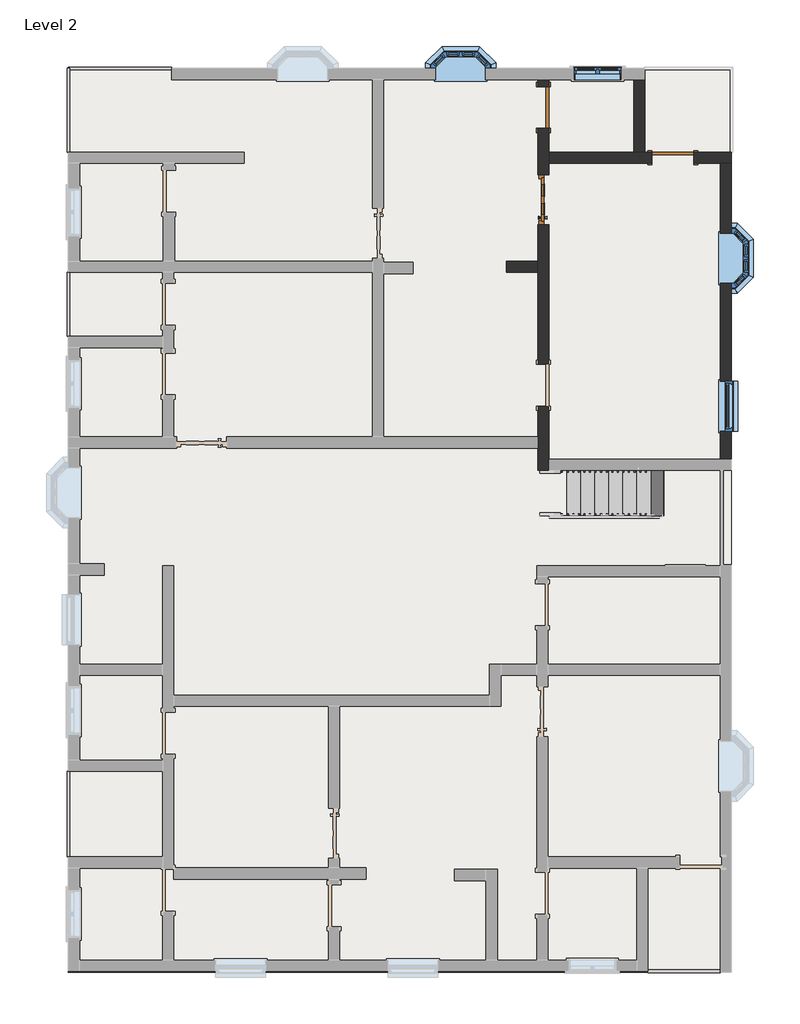
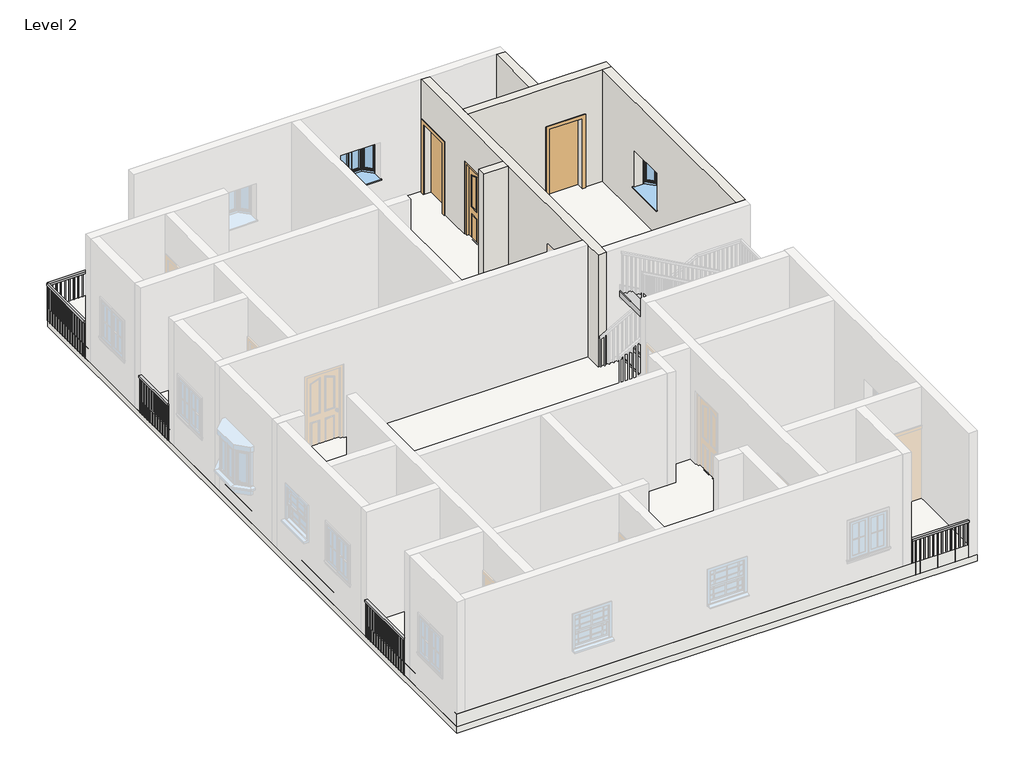
# One storey, part 2 of 4: 5 railings, 5 walls, 4 windows, 3 doors, 1 roof, 1 slab, 1 stair flight.
"""IFC4 building model written with IfcOpenShell, lengths in millimetres."""

from ifc_helpers import new_model, si_unit, frame, origin, place, context, project, spatial, polyline, outline, extrude, faceted_brep, transform, mapped, element, save
from components import doors_extsgl_12_910x2110mm_9a09825e, door_53b1b562, stair_flight_04592867, window_910x910mm_67ef725a, window_c29befe5, windows_sash_w_bars_1_910x910mm_b688f793

model = new_model("IFC4")

# Units and contexts
model_context = context("Model", 3, world=origin())
ifc_project = project(units=[si_unit("LENGTHUNIT", "METRE", prefix="MILLI")], contexts=[model_context])

# Site, building, storey
site = spatial("IfcSite", under=ifc_project)
building = spatial("IfcBuilding", under=site)
storey = spatial("IfcBuildingStorey", under=building, Name="Level 2", Elevation=3048.0)

# Doors
placement = place(None, origin())
doors_extsgl_12_910x2110mm_shape = doors_extsgl_12_910x2110mm_9a09825e(model_context)
element("IfcDoor", 1, ObjectType="Doors_ExtSgl_12 : 910x2110mm", at=placement, inside=storey, context=model_context, shape_type="MappedRepresentation", body=[
    mapped(doors_extsgl_12_910x2110mm_shape, transform((1600.6941283, 5934.0547293, 3048.0), x_axis=(0.0, 1.0, 0.0), y_axis=(-1.0, 0.0, 0.0), z_axis=(0.0, 0.0, 1.0))),
])
door_shape = door_53b1b562(model_context)
element("IfcDoor", 2, ObjectType="Single-Flush : 30\" x 80\"", at=placement, inside=storey, context=model_context, shape_type="MappedRepresentation", body=[
    mapped(door_shape, transform((1600.6941283, 7610.4547293, 3048.0), x_axis=(0.0, 1.0, 0.0), y_axis=(-1.0, 0.0, 0.0), z_axis=(0.0, 0.0, 1.0))),
])
element("IfcDoor", 3, ObjectType="Single-Flush : 30\" x 80\"", at=placement, inside=storey, context=model_context, shape_type="MappedRepresentation", body=[
    mapped(door_shape, transform((3962.8941283, 6696.0547293, 3048.0), x_axis=(-1.0, 0.0, 0.0), y_axis=(0.0, -1.0, 0.0), z_axis=(0.0, 0.0, 1.0))),
])

# Railings
element("IfcRailing", 4, ObjectType="Handrail - Rectangular", at=placement, inside=storey, context=model_context, shape_type="SweptSolid", body=[
    extrude(outline(polyline([(-7073.4058717, 4609.0339901), (-7022.6058717, 4609.0339901), (-7022.6058717, 3444.8547293), (-7073.4058717, 3444.8547293), (-7073.4058717, 4609.0339901)])), frame((0.0, 0.0, 3911.6), z_axis=(0.0, 0.0, 1.0), x_axis=(1.0, 0.0, 0.0)), (0.0, 0.0, 1.0), 50.8),
    extrude(outline(polyline([(-7057.5308717, 3500.9589901), (-7038.4808717, 3500.9589901), (-7038.4808717, 3481.9089901), (-7057.5308717, 3481.9089901), (-7057.5308717, 3500.9589901)])), frame((0.0, 0.0, 3048.0), z_axis=(0.0, 0.0, 1.0), x_axis=(1.0, 0.0, 0.0)), (0.0, 0.0, 1.0), 863.6),
    extrude(outline(polyline([(-7057.5308717, 3602.5589901), (-7038.4808717, 3602.5589901), (-7038.4808717, 3583.5089901), (-7057.5308717, 3583.5089901), (-7057.5308717, 3602.5589901)])), frame((0.0, 0.0, 3048.0), z_axis=(0.0, 0.0, 1.0), x_axis=(1.0, 0.0, 0.0)), (0.0, 0.0, 1.0), 863.6),
    extrude(outline(polyline([(-7057.5308717, 3704.1589901), (-7038.4808717, 3704.1589901), (-7038.4808717, 3685.1089901), (-7057.5308717, 3685.1089901), (-7057.5308717, 3704.1589901)])), frame((0.0, 0.0, 3048.0), z_axis=(0.0, 0.0, 1.0), x_axis=(1.0, 0.0, 0.0)), (0.0, 0.0, 1.0), 863.6),
    extrude(outline(polyline([(-7057.5308717, 3805.7589901), (-7038.4808717, 3805.7589901), (-7038.4808717, 3786.7089901), (-7057.5308717, 3786.7089901), (-7057.5308717, 3805.7589901)])), frame((0.0, 0.0, 3048.0), z_axis=(0.0, 0.0, 1.0), x_axis=(1.0, 0.0, 0.0)), (0.0, 0.0, 1.0), 863.6),
    extrude(outline(polyline([(-7057.5308717, 3907.3589901), (-7038.4808717, 3907.3589901), (-7038.4808717, 3888.3089901), (-7057.5308717, 3888.3089901), (-7057.5308717, 3907.3589901)])), frame((0.0, 0.0, 3048.0), z_axis=(0.0, 0.0, 1.0), x_axis=(1.0, 0.0, 0.0)), (0.0, 0.0, 1.0), 863.6),
    extrude(outline(polyline([(-7057.5308717, 4008.9589901), (-7038.4808717, 4008.9589901), (-7038.4808717, 3989.9089901), (-7057.5308717, 3989.9089901), (-7057.5308717, 4008.9589901)])), frame((0.0, 0.0, 3048.0), z_axis=(0.0, 0.0, 1.0), x_axis=(1.0, 0.0, 0.0)), (0.0, 0.0, 1.0), 863.6),
    extrude(outline(polyline([(-7057.5308717, 4110.5589901), (-7038.4808717, 4110.5589901), (-7038.4808717, 4091.5089901), (-7057.5308717, 4091.5089901), (-7057.5308717, 4110.5589901)])), frame((0.0, 0.0, 3048.0), z_axis=(0.0, 0.0, 1.0), x_axis=(1.0, 0.0, 0.0)), (0.0, 0.0, 1.0), 863.6),
    extrude(outline(polyline([(-7057.5308717, 4212.1589901), (-7038.4808717, 4212.1589901), (-7038.4808717, 4193.1089901), (-7057.5308717, 4193.1089901), (-7057.5308717, 4212.1589901)])), frame((0.0, 0.0, 3048.0), z_axis=(0.0, 0.0, 1.0), x_axis=(1.0, 0.0, 0.0)), (0.0, 0.0, 1.0), 863.6),
    extrude(outline(polyline([(-7057.5308717, 4313.7589901), (-7038.4808717, 4313.7589901), (-7038.4808717, 4294.7089901), (-7057.5308717, 4294.7089901), (-7057.5308717, 4313.7589901)])), frame((0.0, 0.0, 3048.0), z_axis=(0.0, 0.0, 1.0), x_axis=(1.0, 0.0, 0.0)), (0.0, 0.0, 1.0), 863.6),
    extrude(outline(polyline([(-7057.5308717, 4415.3589901), (-7038.4808717, 4415.3589901), (-7038.4808717, 4396.3089901), (-7057.5308717, 4396.3089901), (-7057.5308717, 4415.3589901)])), frame((0.0, 0.0, 3048.0), z_axis=(0.0, 0.0, 1.0), x_axis=(1.0, 0.0, 0.0)), (0.0, 0.0, 1.0), 863.6),
    extrude(outline(polyline([(-7057.5308717, 4516.9589901), (-7038.4808717, 4516.9589901), (-7038.4808717, 4497.9089901), (-7057.5308717, 4497.9089901), (-7057.5308717, 4516.9589901)])), frame((0.0, 0.0, 3048.0), z_axis=(0.0, 0.0, 1.0), x_axis=(1.0, 0.0, 0.0)), (0.0, 0.0, 1.0), 863.6),
    extrude(outline(polyline([(-7057.5308717, 3463.9047293), (-7038.4808717, 3463.9047293), (-7038.4808717, 3444.8547293), (-7057.5308717, 3444.8547293), (-7057.5308717, 3463.9047293)])), frame((0.0, 0.0, 3048.0), z_axis=(0.0, 0.0, 1.0), x_axis=(1.0, 0.0, 0.0)), (0.0, 0.0, 1.0), 863.6),
    extrude(outline(polyline([(-7057.5308717, 4609.0339901), (-7038.4808717, 4609.0339901), (-7038.4808717, 4589.9839901), (-7057.5308717, 4589.9839901), (-7057.5308717, 4609.0339901)])), frame((0.0, 0.0, 3048.0), z_axis=(0.0, 0.0, 1.0), x_axis=(1.0, 0.0, 0.0)), (0.0, 0.0, 1.0), 863.6),
])
element("IfcRailing", 5, ObjectType="Handrail - Rectangular", at=placement, inside=storey, context=model_context, shape_type="SweptSolid", body=[
    extrude(outline(polyline([(-7073.4058717, -4474.6886333), (-7022.6058717, -4474.6886333), (-7022.6058717, -6029.3452707), (-7073.4058717, -6029.3452707), (-7073.4058717, -4474.6886333)])), frame((0.0, 0.0, 3911.6), z_axis=(0.0, 0.0, 1.0), x_axis=(1.0, 0.0, 0.0)), (0.0, 0.0, 1.0), 50.8),
    extrude(outline(polyline([(-7057.5308717, -5989.1636333), (-7038.4808717, -5989.1636333), (-7038.4808717, -6008.2136333), (-7057.5308717, -6008.2136333), (-7057.5308717, -5989.1636333)])), frame((0.0, 0.0, 3048.0), z_axis=(0.0, 0.0, 1.0), x_axis=(1.0, 0.0, 0.0)), (0.0, 0.0, 1.0), 863.6),
    extrude(outline(polyline([(-7057.5308717, -5887.5636333), (-7038.4808717, -5887.5636333), (-7038.4808717, -5906.6136333), (-7057.5308717, -5906.6136333), (-7057.5308717, -5887.5636333)])), frame((0.0, 0.0, 3048.0), z_axis=(0.0, 0.0, 1.0), x_axis=(1.0, 0.0, 0.0)), (0.0, 0.0, 1.0), 863.6),
    extrude(outline(polyline([(-7057.5308717, -5785.9636333), (-7038.4808717, -5785.9636333), (-7038.4808717, -5805.0136333), (-7057.5308717, -5805.0136333), (-7057.5308717, -5785.9636333)])), frame((0.0, 0.0, 3048.0), z_axis=(0.0, 0.0, 1.0), x_axis=(1.0, 0.0, 0.0)), (0.0, 0.0, 1.0), 863.6),
    extrude(outline(polyline([(-7057.5308717, -5684.3636333), (-7038.4808717, -5684.3636333), (-7038.4808717, -5703.4136333), (-7057.5308717, -5703.4136333), (-7057.5308717, -5684.3636333)])), frame((0.0, 0.0, 3048.0), z_axis=(0.0, 0.0, 1.0), x_axis=(1.0, 0.0, 0.0)), (0.0, 0.0, 1.0), 863.6),
    extrude(outline(polyline([(-7057.5308717, -5582.7636333), (-7038.4808717, -5582.7636333), (-7038.4808717, -5601.8136333), (-7057.5308717, -5601.8136333), (-7057.5308717, -5582.7636333)])), frame((0.0, 0.0, 3048.0), z_axis=(0.0, 0.0, 1.0), x_axis=(1.0, 0.0, 0.0)), (0.0, 0.0, 1.0), 863.6),
    extrude(outline(polyline([(-7057.5308717, -5481.1636333), (-7038.4808717, -5481.1636333), (-7038.4808717, -5500.2136333), (-7057.5308717, -5500.2136333), (-7057.5308717, -5481.1636333)])), frame((0.0, 0.0, 3048.0), z_axis=(0.0, 0.0, 1.0), x_axis=(1.0, 0.0, 0.0)), (0.0, 0.0, 1.0), 863.6),
    extrude(outline(polyline([(-7057.5308717, -5379.5636333), (-7038.4808717, -5379.5636333), (-7038.4808717, -5398.6136333), (-7057.5308717, -5398.6136333), (-7057.5308717, -5379.5636333)])), frame((0.0, 0.0, 3048.0), z_axis=(0.0, 0.0, 1.0), x_axis=(1.0, 0.0, 0.0)), (0.0, 0.0, 1.0), 863.6),
    extrude(outline(polyline([(-7057.5308717, -5277.9636333), (-7038.4808717, -5277.9636333), (-7038.4808717, -5297.0136333), (-7057.5308717, -5297.0136333), (-7057.5308717, -5277.9636333)])), frame((0.0, 0.0, 3048.0), z_axis=(0.0, 0.0, 1.0), x_axis=(1.0, 0.0, 0.0)), (0.0, 0.0, 1.0), 863.6),
    extrude(outline(polyline([(-7057.5308717, -5176.3636333), (-7038.4808717, -5176.3636333), (-7038.4808717, -5195.4136333), (-7057.5308717, -5195.4136333), (-7057.5308717, -5176.3636333)])), frame((0.0, 0.0, 3048.0), z_axis=(0.0, 0.0, 1.0), x_axis=(1.0, 0.0, 0.0)), (0.0, 0.0, 1.0), 863.6),
    extrude(outline(polyline([(-7057.5308717, -5074.7636333), (-7038.4808717, -5074.7636333), (-7038.4808717, -5093.8136333), (-7057.5308717, -5093.8136333), (-7057.5308717, -5074.7636333)])), frame((0.0, 0.0, 3048.0), z_axis=(0.0, 0.0, 1.0), x_axis=(1.0, 0.0, 0.0)), (0.0, 0.0, 1.0), 863.6),
    extrude(outline(polyline([(-7057.5308717, -4973.1636333), (-7038.4808717, -4973.1636333), (-7038.4808717, -4992.2136333), (-7057.5308717, -4992.2136333), (-7057.5308717, -4973.1636333)])), frame((0.0, 0.0, 3048.0), z_axis=(0.0, 0.0, 1.0), x_axis=(1.0, 0.0, 0.0)), (0.0, 0.0, 1.0), 863.6),
    extrude(outline(polyline([(-7057.5308717, -4871.5636333), (-7038.4808717, -4871.5636333), (-7038.4808717, -4890.6136333), (-7057.5308717, -4890.6136333), (-7057.5308717, -4871.5636333)])), frame((0.0, 0.0, 3048.0), z_axis=(0.0, 0.0, 1.0), x_axis=(1.0, 0.0, 0.0)), (0.0, 0.0, 1.0), 863.6),
    extrude(outline(polyline([(-7057.5308717, -4769.9636333), (-7038.4808717, -4769.9636333), (-7038.4808717, -4789.0136333), (-7057.5308717, -4789.0136333), (-7057.5308717, -4769.9636333)])), frame((0.0, 0.0, 3048.0), z_axis=(0.0, 0.0, 1.0), x_axis=(1.0, 0.0, 0.0)), (0.0, 0.0, 1.0), 863.6),
    extrude(outline(polyline([(-7057.5308717, -4668.3636333), (-7038.4808717, -4668.3636333), (-7038.4808717, -4687.4136333), (-7057.5308717, -4687.4136333), (-7057.5308717, -4668.3636333)])), frame((0.0, 0.0, 3048.0), z_axis=(0.0, 0.0, 1.0), x_axis=(1.0, 0.0, 0.0)), (0.0, 0.0, 1.0), 863.6),
    extrude(outline(polyline([(-7057.5308717, -4566.7636333), (-7038.4808717, -4566.7636333), (-7038.4808717, -4585.8136333), (-7057.5308717, -4585.8136333), (-7057.5308717, -4566.7636333)])), frame((0.0, 0.0, 3048.0), z_axis=(0.0, 0.0, 1.0), x_axis=(1.0, 0.0, 0.0)), (0.0, 0.0, 1.0), 863.6),
    extrude(outline(polyline([(-7057.5308717, -6010.2952707), (-7038.4808717, -6010.2952707), (-7038.4808717, -6029.3452707), (-7057.5308717, -6029.3452707), (-7057.5308717, -6010.2952707)])), frame((0.0, 0.0, 3048.0), z_axis=(0.0, 0.0, 1.0), x_axis=(1.0, 0.0, 0.0)), (0.0, 0.0, 1.0), 863.6),
    extrude(outline(polyline([(-7057.5308717, -4474.6886333), (-7038.4808717, -4474.6886333), (-7038.4808717, -4493.7386333), (-7057.5308717, -4493.7386333), (-7057.5308717, -4474.6886333)])), frame((0.0, 0.0, 3048.0), z_axis=(0.0, 0.0, 1.0), x_axis=(1.0, 0.0, 0.0)), (0.0, 0.0, 1.0), 863.6),
])
element("IfcRailing", 6, ObjectType="Handrail - Rectangular", at=placement, inside=storey, context=model_context, shape_type="SweptSolid", body=[
    extrude(outline(polyline([(3505.6941283, -8137.5452707), (3505.6941283, -8086.7452707), (4826.4941283, -8086.7452707), (4826.4941283, -8137.5452707), (3505.6941283, -8137.5452707)])), frame((0.0, 0.0, 3911.6), z_axis=(0.0, 0.0, 1.0), x_axis=(1.0, 0.0, 0.0)), (0.0, 0.0, 1.0), 50.8),
    extrude(outline(polyline([(4715.3691283, -8121.6702707), (4715.3691283, -8102.6202707), (4734.4191283, -8102.6202707), (4734.4191283, -8121.6702707), (4715.3691283, -8121.6702707)])), frame((0.0, 0.0, 3048.0), z_axis=(0.0, 0.0, 1.0), x_axis=(1.0, 0.0, 0.0)), (0.0, 0.0, 1.0), 863.6),
    extrude(outline(polyline([(4613.7691283, -8121.6702707), (4613.7691283, -8102.6202707), (4632.8191283, -8102.6202707), (4632.8191283, -8121.6702707), (4613.7691283, -8121.6702707)])), frame((0.0, 0.0, 3048.0), z_axis=(0.0, 0.0, 1.0), x_axis=(1.0, 0.0, 0.0)), (0.0, 0.0, 1.0), 863.6),
    extrude(outline(polyline([(4512.1691283, -8121.6702707), (4512.1691283, -8102.6202707), (4531.2191283, -8102.6202707), (4531.2191283, -8121.6702707), (4512.1691283, -8121.6702707)])), frame((0.0, 0.0, 3048.0), z_axis=(0.0, 0.0, 1.0), x_axis=(1.0, 0.0, 0.0)), (0.0, 0.0, 1.0), 863.6),
    extrude(outline(polyline([(4410.5691283, -8121.6702707), (4410.5691283, -8102.6202707), (4429.6191283, -8102.6202707), (4429.6191283, -8121.6702707), (4410.5691283, -8121.6702707)])), frame((0.0, 0.0, 3048.0), z_axis=(0.0, 0.0, 1.0), x_axis=(1.0, 0.0, 0.0)), (0.0, 0.0, 1.0), 863.6),
    extrude(outline(polyline([(4308.9691283, -8121.6702707), (4308.9691283, -8102.6202707), (4328.0191283, -8102.6202707), (4328.0191283, -8121.6702707), (4308.9691283, -8121.6702707)])), frame((0.0, 0.0, 3048.0), z_axis=(0.0, 0.0, 1.0), x_axis=(1.0, 0.0, 0.0)), (0.0, 0.0, 1.0), 863.6),
    extrude(outline(polyline([(4207.3691283, -8121.6702707), (4207.3691283, -8102.6202707), (4226.4191283, -8102.6202707), (4226.4191283, -8121.6702707), (4207.3691283, -8121.6702707)])), frame((0.0, 0.0, 3048.0), z_axis=(0.0, 0.0, 1.0), x_axis=(1.0, 0.0, 0.0)), (0.0, 0.0, 1.0), 863.6),
    extrude(outline(polyline([(4105.7691283, -8121.6702707), (4105.7691283, -8102.6202707), (4124.8191283, -8102.6202707), (4124.8191283, -8121.6702707), (4105.7691283, -8121.6702707)])), frame((0.0, 0.0, 3048.0), z_axis=(0.0, 0.0, 1.0), x_axis=(1.0, 0.0, 0.0)), (0.0, 0.0, 1.0), 863.6),
    extrude(outline(polyline([(4004.1691283, -8121.6702707), (4004.1691283, -8102.6202707), (4023.2191283, -8102.6202707), (4023.2191283, -8121.6702707), (4004.1691283, -8121.6702707)])), frame((0.0, 0.0, 3048.0), z_axis=(0.0, 0.0, 1.0), x_axis=(1.0, 0.0, 0.0)), (0.0, 0.0, 1.0), 863.6),
    extrude(outline(polyline([(3902.5691283, -8121.6702707), (3902.5691283, -8102.6202707), (3921.6191283, -8102.6202707), (3921.6191283, -8121.6702707), (3902.5691283, -8121.6702707)])), frame((0.0, 0.0, 3048.0), z_axis=(0.0, 0.0, 1.0), x_axis=(1.0, 0.0, 0.0)), (0.0, 0.0, 1.0), 863.6),
    extrude(outline(polyline([(3800.9691283, -8121.6702707), (3800.9691283, -8102.6202707), (3820.0191283, -8102.6202707), (3820.0191283, -8121.6702707), (3800.9691283, -8121.6702707)])), frame((0.0, 0.0, 3048.0), z_axis=(0.0, 0.0, 1.0), x_axis=(1.0, 0.0, 0.0)), (0.0, 0.0, 1.0), 863.6),
    extrude(outline(polyline([(3699.3691283, -8121.6702707), (3699.3691283, -8102.6202707), (3718.4191283, -8102.6202707), (3718.4191283, -8121.6702707), (3699.3691283, -8121.6702707)])), frame((0.0, 0.0, 3048.0), z_axis=(0.0, 0.0, 1.0), x_axis=(1.0, 0.0, 0.0)), (0.0, 0.0, 1.0), 863.6),
    extrude(outline(polyline([(3597.7691283, -8121.6702707), (3597.7691283, -8102.6202707), (3616.8191283, -8102.6202707), (3616.8191283, -8121.6702707), (3597.7691283, -8121.6702707)])), frame((0.0, 0.0, 3048.0), z_axis=(0.0, 0.0, 1.0), x_axis=(1.0, 0.0, 0.0)), (0.0, 0.0, 1.0), 863.6),
    extrude(outline(polyline([(4807.4441283, -8121.6702707), (4807.4441283, -8102.6202707), (4826.4941283, -8102.6202707), (4826.4941283, -8121.6702707), (4807.4441283, -8121.6702707)])), frame((0.0, 0.0, 3048.0), z_axis=(0.0, 0.0, 1.0), x_axis=(1.0, 0.0, 0.0)), (0.0, 0.0, 1.0), 863.6),
    extrude(outline(polyline([(3505.6941283, -8121.6702707), (3505.6941283, -8102.6202707), (3524.7441283, -8102.6202707), (3524.7441283, -8121.6702707), (3505.6941283, -8121.6702707)])), frame((0.0, 0.0, 3048.0), z_axis=(0.0, 0.0, 1.0), x_axis=(1.0, 0.0, 0.0)), (0.0, 0.0, 1.0), 863.6),
])
element("IfcRailing", 7, ObjectType="Handrail - Rectangular", at=placement, inside=storey, context=model_context, shape_type="SweptSolid", body=[
    extrude(outline(polyline([(-7022.6058717, 6797.6547293), (-7073.4058717, 6797.6547293), (-7073.4058717, 8321.6547293), (-7022.6058717, 8321.6547293), (-7022.6058717, 6797.6547293)])), frame((0.0, 0.0, 3911.6), z_axis=(0.0, 0.0, 1.0), x_axis=(1.0, 0.0, 0.0)), (0.0, 0.0, 1.0), 50.8),
    extrude(outline(polyline([(-7038.4808717, 8210.5297293), (-7057.5308717, 8210.5297293), (-7057.5308717, 8229.5797293), (-7038.4808717, 8229.5797293), (-7038.4808717, 8210.5297293)])), frame((0.0, 0.0, 3048.0), z_axis=(0.0, 0.0, 1.0), x_axis=(1.0, 0.0, 0.0)), (0.0, 0.0, 1.0), 863.6),
    extrude(outline(polyline([(-7038.4808717, 8108.9297293), (-7057.5308717, 8108.9297293), (-7057.5308717, 8127.9797293), (-7038.4808717, 8127.9797293), (-7038.4808717, 8108.9297293)])), frame((0.0, 0.0, 3048.0), z_axis=(0.0, 0.0, 1.0), x_axis=(1.0, 0.0, 0.0)), (0.0, 0.0, 1.0), 863.6),
    extrude(outline(polyline([(-7038.4808717, 8007.3297293), (-7057.5308717, 8007.3297293), (-7057.5308717, 8026.3797293), (-7038.4808717, 8026.3797293), (-7038.4808717, 8007.3297293)])), frame((0.0, 0.0, 3048.0), z_axis=(0.0, 0.0, 1.0), x_axis=(1.0, 0.0, 0.0)), (0.0, 0.0, 1.0), 863.6),
    extrude(outline(polyline([(-7038.4808717, 7905.7297293), (-7057.5308717, 7905.7297293), (-7057.5308717, 7924.7797293), (-7038.4808717, 7924.7797293), (-7038.4808717, 7905.7297293)])), frame((0.0, 0.0, 3048.0), z_axis=(0.0, 0.0, 1.0), x_axis=(1.0, 0.0, 0.0)), (0.0, 0.0, 1.0), 863.6),
    extrude(outline(polyline([(-7038.4808717, 7804.1297293), (-7057.5308717, 7804.1297293), (-7057.5308717, 7823.1797293), (-7038.4808717, 7823.1797293), (-7038.4808717, 7804.1297293)])), frame((0.0, 0.0, 3048.0), z_axis=(0.0, 0.0, 1.0), x_axis=(1.0, 0.0, 0.0)), (0.0, 0.0, 1.0), 863.6),
    extrude(outline(polyline([(-7038.4808717, 7702.5297293), (-7057.5308717, 7702.5297293), (-7057.5308717, 7721.5797293), (-7038.4808717, 7721.5797293), (-7038.4808717, 7702.5297293)])), frame((0.0, 0.0, 3048.0), z_axis=(0.0, 0.0, 1.0), x_axis=(1.0, 0.0, 0.0)), (0.0, 0.0, 1.0), 863.6),
    extrude(outline(polyline([(-7038.4808717, 7600.9297293), (-7057.5308717, 7600.9297293), (-7057.5308717, 7619.9797293), (-7038.4808717, 7619.9797293), (-7038.4808717, 7600.9297293)])), frame((0.0, 0.0, 3048.0), z_axis=(0.0, 0.0, 1.0), x_axis=(1.0, 0.0, 0.0)), (0.0, 0.0, 1.0), 863.6),
    extrude(outline(polyline([(-7038.4808717, 7499.3297293), (-7057.5308717, 7499.3297293), (-7057.5308717, 7518.3797293), (-7038.4808717, 7518.3797293), (-7038.4808717, 7499.3297293)])), frame((0.0, 0.0, 3048.0), z_axis=(0.0, 0.0, 1.0), x_axis=(1.0, 0.0, 0.0)), (0.0, 0.0, 1.0), 863.6),
    extrude(outline(polyline([(-7038.4808717, 7397.7297293), (-7057.5308717, 7397.7297293), (-7057.5308717, 7416.7797293), (-7038.4808717, 7416.7797293), (-7038.4808717, 7397.7297293)])), frame((0.0, 0.0, 3048.0), z_axis=(0.0, 0.0, 1.0), x_axis=(1.0, 0.0, 0.0)), (0.0, 0.0, 1.0), 863.6),
    extrude(outline(polyline([(-7038.4808717, 7296.1297293), (-7057.5308717, 7296.1297293), (-7057.5308717, 7315.1797293), (-7038.4808717, 7315.1797293), (-7038.4808717, 7296.1297293)])), frame((0.0, 0.0, 3048.0), z_axis=(0.0, 0.0, 1.0), x_axis=(1.0, 0.0, 0.0)), (0.0, 0.0, 1.0), 863.6),
    extrude(outline(polyline([(-7038.4808717, 7194.5297293), (-7057.5308717, 7194.5297293), (-7057.5308717, 7213.5797293), (-7038.4808717, 7213.5797293), (-7038.4808717, 7194.5297293)])), frame((0.0, 0.0, 3048.0), z_axis=(0.0, 0.0, 1.0), x_axis=(1.0, 0.0, 0.0)), (0.0, 0.0, 1.0), 863.6),
    extrude(outline(polyline([(-7038.4808717, 7092.9297293), (-7057.5308717, 7092.9297293), (-7057.5308717, 7111.9797293), (-7038.4808717, 7111.9797293), (-7038.4808717, 7092.9297293)])), frame((0.0, 0.0, 3048.0), z_axis=(0.0, 0.0, 1.0), x_axis=(1.0, 0.0, 0.0)), (0.0, 0.0, 1.0), 863.6),
    extrude(outline(polyline([(-7038.4808717, 6991.3297293), (-7057.5308717, 6991.3297293), (-7057.5308717, 7010.3797293), (-7038.4808717, 7010.3797293), (-7038.4808717, 6991.3297293)])), frame((0.0, 0.0, 3048.0), z_axis=(0.0, 0.0, 1.0), x_axis=(1.0, 0.0, 0.0)), (0.0, 0.0, 1.0), 863.6),
    extrude(outline(polyline([(-7038.4808717, 6889.7297293), (-7057.5308717, 6889.7297293), (-7057.5308717, 6908.7797293), (-7038.4808717, 6908.7797293), (-7038.4808717, 6889.7297293)])), frame((0.0, 0.0, 3048.0), z_axis=(0.0, 0.0, 1.0), x_axis=(1.0, 0.0, 0.0)), (0.0, 0.0, 1.0), 863.6),
    extrude(outline(polyline([(-7038.4808717, 8302.6047293), (-7057.5308717, 8302.6047293), (-7057.5308717, 8321.6547293), (-7038.4808717, 8321.6547293), (-7038.4808717, 8302.6047293)])), frame((0.0, 0.0, 3048.0), z_axis=(0.0, 0.0, 1.0), x_axis=(1.0, 0.0, 0.0)), (0.0, 0.0, 1.0), 863.6),
    extrude(outline(polyline([(-7038.4808717, 6797.6547293), (-7057.5308717, 6797.6547293), (-7057.5308717, 6816.7047293), (-7038.4808717, 6816.7047293), (-7038.4808717, 6797.6547293)])), frame((0.0, 0.0, 3048.0), z_axis=(0.0, 0.0, 1.0), x_axis=(1.0, 0.0, 0.0)), (0.0, 0.0, 1.0), 863.6),
])
element("IfcRailing", 8, ObjectType="Handrail - Rectangular", at=placement, inside=storey, context=model_context, shape_type="SweptSolid", body=[
    extrude(outline(polyline([(-7048.0058717, 8296.2547293), (-7048.0058717, 8347.0547293), (-5168.4058717, 8347.0547293), (-5168.4058717, 8296.2547293), (-7048.0058717, 8296.2547293)])), frame((0.0, 0.0, 3911.6), z_axis=(0.0, 0.0, 1.0), x_axis=(1.0, 0.0, 0.0)), (0.0, 0.0, 1.0), 50.8),
    extrude(outline(polyline([(-5228.7308717, 8312.1297293), (-5228.7308717, 8331.1797293), (-5209.6808717, 8331.1797293), (-5209.6808717, 8312.1297293), (-5228.7308717, 8312.1297293)])), frame((0.0, 0.0, 3048.0), z_axis=(0.0, 0.0, 1.0), x_axis=(1.0, 0.0, 0.0)), (0.0, 0.0, 1.0), 863.6),
    extrude(outline(polyline([(-5330.3308717, 8312.1297293), (-5330.3308717, 8331.1797293), (-5311.2808717, 8331.1797293), (-5311.2808717, 8312.1297293), (-5330.3308717, 8312.1297293)])), frame((0.0, 0.0, 3048.0), z_axis=(0.0, 0.0, 1.0), x_axis=(1.0, 0.0, 0.0)), (0.0, 0.0, 1.0), 863.6),
    extrude(outline(polyline([(-5431.9308717, 8312.1297293), (-5431.9308717, 8331.1797293), (-5412.8808717, 8331.1797293), (-5412.8808717, 8312.1297293), (-5431.9308717, 8312.1297293)])), frame((0.0, 0.0, 3048.0), z_axis=(0.0, 0.0, 1.0), x_axis=(1.0, 0.0, 0.0)), (0.0, 0.0, 1.0), 863.6),
    extrude(outline(polyline([(-5533.5308717, 8312.1297293), (-5533.5308717, 8331.1797293), (-5514.4808717, 8331.1797293), (-5514.4808717, 8312.1297293), (-5533.5308717, 8312.1297293)])), frame((0.0, 0.0, 3048.0), z_axis=(0.0, 0.0, 1.0), x_axis=(1.0, 0.0, 0.0)), (0.0, 0.0, 1.0), 863.6),
    extrude(outline(polyline([(-5635.1308717, 8312.1297293), (-5635.1308717, 8331.1797293), (-5616.0808717, 8331.1797293), (-5616.0808717, 8312.1297293), (-5635.1308717, 8312.1297293)])), frame((0.0, 0.0, 3048.0), z_axis=(0.0, 0.0, 1.0), x_axis=(1.0, 0.0, 0.0)), (0.0, 0.0, 1.0), 863.6),
    extrude(outline(polyline([(-5736.7308717, 8312.1297293), (-5736.7308717, 8331.1797293), (-5717.6808717, 8331.1797293), (-5717.6808717, 8312.1297293), (-5736.7308717, 8312.1297293)])), frame((0.0, 0.0, 3048.0), z_axis=(0.0, 0.0, 1.0), x_axis=(1.0, 0.0, 0.0)), (0.0, 0.0, 1.0), 863.6),
    extrude(outline(polyline([(-5838.3308717, 8312.1297293), (-5838.3308717, 8331.1797293), (-5819.2808717, 8331.1797293), (-5819.2808717, 8312.1297293), (-5838.3308717, 8312.1297293)])), frame((0.0, 0.0, 3048.0), z_axis=(0.0, 0.0, 1.0), x_axis=(1.0, 0.0, 0.0)), (0.0, 0.0, 1.0), 863.6),
    extrude(outline(polyline([(-5939.9308717, 8312.1297293), (-5939.9308717, 8331.1797293), (-5920.8808717, 8331.1797293), (-5920.8808717, 8312.1297293), (-5939.9308717, 8312.1297293)])), frame((0.0, 0.0, 3048.0), z_axis=(0.0, 0.0, 1.0), x_axis=(1.0, 0.0, 0.0)), (0.0, 0.0, 1.0), 863.6),
    extrude(outline(polyline([(-6041.5308717, 8312.1297293), (-6041.5308717, 8331.1797293), (-6022.4808717, 8331.1797293), (-6022.4808717, 8312.1297293), (-6041.5308717, 8312.1297293)])), frame((0.0, 0.0, 3048.0), z_axis=(0.0, 0.0, 1.0), x_axis=(1.0, 0.0, 0.0)), (0.0, 0.0, 1.0), 863.6),
    extrude(outline(polyline([(-6143.1308717, 8312.1297293), (-6143.1308717, 8331.1797293), (-6124.0808717, 8331.1797293), (-6124.0808717, 8312.1297293), (-6143.1308717, 8312.1297293)])), frame((0.0, 0.0, 3048.0), z_axis=(0.0, 0.0, 1.0), x_axis=(1.0, 0.0, 0.0)), (0.0, 0.0, 1.0), 863.6),
    extrude(outline(polyline([(-6244.7308717, 8312.1297293), (-6244.7308717, 8331.1797293), (-6225.6808717, 8331.1797293), (-6225.6808717, 8312.1297293), (-6244.7308717, 8312.1297293)])), frame((0.0, 0.0, 3048.0), z_axis=(0.0, 0.0, 1.0), x_axis=(1.0, 0.0, 0.0)), (0.0, 0.0, 1.0), 863.6),
    extrude(outline(polyline([(-6346.3308717, 8312.1297293), (-6346.3308717, 8331.1797293), (-6327.2808717, 8331.1797293), (-6327.2808717, 8312.1297293), (-6346.3308717, 8312.1297293)])), frame((0.0, 0.0, 3048.0), z_axis=(0.0, 0.0, 1.0), x_axis=(1.0, 0.0, 0.0)), (0.0, 0.0, 1.0), 863.6),
    extrude(outline(polyline([(-6447.9308717, 8312.1297293), (-6447.9308717, 8331.1797293), (-6428.8808717, 8331.1797293), (-6428.8808717, 8312.1297293), (-6447.9308717, 8312.1297293)])), frame((0.0, 0.0, 3048.0), z_axis=(0.0, 0.0, 1.0), x_axis=(1.0, 0.0, 0.0)), (0.0, 0.0, 1.0), 863.6),
    extrude(outline(polyline([(-6549.5308717, 8312.1297293), (-6549.5308717, 8331.1797293), (-6530.4808717, 8331.1797293), (-6530.4808717, 8312.1297293), (-6549.5308717, 8312.1297293)])), frame((0.0, 0.0, 3048.0), z_axis=(0.0, 0.0, 1.0), x_axis=(1.0, 0.0, 0.0)), (0.0, 0.0, 1.0), 863.6),
    extrude(outline(polyline([(-6651.1308717, 8312.1297293), (-6651.1308717, 8331.1797293), (-6632.0808717, 8331.1797293), (-6632.0808717, 8312.1297293), (-6651.1308717, 8312.1297293)])), frame((0.0, 0.0, 3048.0), z_axis=(0.0, 0.0, 1.0), x_axis=(1.0, 0.0, 0.0)), (0.0, 0.0, 1.0), 863.6),
    extrude(outline(polyline([(-6752.7308717, 8312.1297293), (-6752.7308717, 8331.1797293), (-6733.6808717, 8331.1797293), (-6733.6808717, 8312.1297293), (-6752.7308717, 8312.1297293)])), frame((0.0, 0.0, 3048.0), z_axis=(0.0, 0.0, 1.0), x_axis=(1.0, 0.0, 0.0)), (0.0, 0.0, 1.0), 863.6),
    extrude(outline(polyline([(-6854.3308717, 8312.1297293), (-6854.3308717, 8331.1797293), (-6835.2808717, 8331.1797293), (-6835.2808717, 8312.1297293), (-6854.3308717, 8312.1297293)])), frame((0.0, 0.0, 3048.0), z_axis=(0.0, 0.0, 1.0), x_axis=(1.0, 0.0, 0.0)), (0.0, 0.0, 1.0), 863.6),
    extrude(outline(polyline([(-6955.9308717, 8312.1297293), (-6955.9308717, 8331.1797293), (-6936.8808717, 8331.1797293), (-6936.8808717, 8312.1297293), (-6955.9308717, 8312.1297293)])), frame((0.0, 0.0, 3048.0), z_axis=(0.0, 0.0, 1.0), x_axis=(1.0, 0.0, 0.0)), (0.0, 0.0, 1.0), 863.6),
    extrude(outline(polyline([(-5187.4558717, 8312.1297293), (-5187.4558717, 8331.1797293), (-5168.4058717, 8331.1797293), (-5168.4058717, 8312.1297293), (-5187.4558717, 8312.1297293)])), frame((0.0, 0.0, 3048.0), z_axis=(0.0, 0.0, 1.0), x_axis=(1.0, 0.0, 0.0)), (0.0, 0.0, 1.0), 863.6),
    extrude(outline(polyline([(-7048.0058717, 8312.1297293), (-7048.0058717, 8331.1797293), (-7028.9558717, 8331.1797293), (-7028.9558717, 8312.1297293), (-7048.0058717, 8312.1297293)])), frame((0.0, 0.0, 3048.0), z_axis=(0.0, 0.0, 1.0), x_axis=(1.0, 0.0, 0.0)), (0.0, 0.0, 1.0), 863.6),
])

# Roof
element("IfcRoof", 9, ObjectType="Generic - 12\"", at=placement, inside=storey, context=model_context, shape_type="SweptSolid", body=[
    extrude(outline(polyline([(-7048.0058717, 8321.6547293), (5029.6941283, 8321.6547293), (5029.6941283, -8124.8452707), (-7048.0058717, -8124.8452707), (-7048.0058717, 8321.6547293)])), frame((0.0, 0.0, 3048.0), z_axis=(0.0, 0.0, 1.0), x_axis=(1.0, 0.0, 0.0)), (0.0, 0.0, 1.0), 304.8),
])

# Slab
element("IfcSlab", 10, ObjectType="Generic - 12\"", at=placement, inside=storey, context=model_context, shape_type="SweptSolid", body=[
    extrude(outline(polyline([(5029.6941283, 8321.6547293), (5029.6941283, -8124.8452707), (-7048.0058717, -8124.8452707), (-7048.0058717, 8321.6547293), (5029.6941283, 8321.6547293)])), frame((0.0, 0.0, 2895.6), z_axis=(0.0, 0.0, 1.0), x_axis=(1.0, 0.0, 0.0)), (0.0, 0.0, 1.0), 152.4),
])

# Stair flight
stair_flight_shape = stair_flight_04592867(model_context)
element("IfcStairFlight", 11, ObjectType="2\" Tread 1\" Nosing 1/4\" Riser", at=placement, inside=storey, context=model_context, shape_type="MappedRepresentation", body=[
    mapped(stair_flight_shape, transform((0.0, 0.0, 0.0), x_axis=(1.0, 0.0, 0.0), y_axis=(0.0, 1.0, 0.0), z_axis=(0.0, 0.0, 1.0))),
])

# Walls
element("IfcWall", 12, ObjectType="Generic - 4.5\"", at=placement, inside=storey, context=model_context, shape_type="Brep", body=[
    faceted_brep([(1499.0941283, 8118.4547293, 3048.0), (1499.0941283, 7991.4547293, 3048.0), (1499.0941283, 7991.4547293, 5080.0), (1499.0941283, 7229.4547293, 5080.0), (1499.0941283, 7229.4547293, 3048.0), (1499.0941283, 6389.0547293, 3048.0), (1499.0941283, 6389.0547293, 5158.0), (1499.0941283, 5479.0547293, 5158.0), (1499.0941283, 5479.0547293, 3048.0), (1499.0941283, 4812.2339901, 3048.0), (1499.0941283, 4609.0339901, 3048.0), (1499.0941283, 2936.8547293, 3048.0), (1499.0941283, 2936.8547293, 5080.0), (1499.0941283, 2174.8547293, 5080.0), (1499.0941283, 2174.8547293, 3048.0), (1499.0941283, 1616.0547293, 3048.0), (1499.0941283, 1412.8547293, 3048.0), (1499.0941283, 1006.4547293, 3048.0), (1499.0941283, 1006.4547293, 6096.0), (1499.0941283, 1412.8547293, 6096.0), (1499.0941283, 1616.0547293, 6096.0), (1499.0941283, 4609.0339901, 6096.0), (1499.0941283, 4812.2339901, 6096.0), (1499.0941283, 8118.4547293, 6096.0), (1702.2941283, 7991.4547293, 5080.0), (1702.2941283, 7991.4547293, 3048.0), (1702.2941283, 8118.4547293, 3048.0), (1702.2941283, 8118.4547293, 6096.0), (1702.2941283, 6797.6547293, 6096.0), (1702.2941283, 6594.4547293, 6096.0), (1702.2941283, 1209.6547293, 6096.0), (1702.2941283, 1006.4547293, 6096.0), (1702.2941283, 1006.4547293, 3048.0), (1702.2941283, 1209.6547293, 3048.0), (1702.2941283, 2174.8547293, 3048.0), (1702.2941283, 2174.8547293, 5080.0), (1702.2941283, 2936.8547293, 5080.0), (1702.2941283, 2936.8547293, 3048.0), (1702.2941283, 5479.0547293, 3048.0), (1702.2941283, 5479.0547293, 5158.0), (1702.2941283, 6389.0547293, 5158.0), (1702.2941283, 6389.0547293, 3048.0), (1702.2941283, 6594.4547293, 3048.0), (1702.2941283, 6797.6547293, 3048.0), (1702.2941283, 7229.4547293, 3048.0), (1702.2941283, 7229.4547293, 5080.0)], [[[0, 1, 2, 3, 4, 5, 6, 7, 8, 9, 10, 11, 12, 13, 14, 15, 16, 17, 18, 19, 20, 21, 22, 23]], [[24, 25, 26, 27, 28, 29, 30, 31, 32, 33, 34, 35, 36, 37, 38, 39, 40, 41, 42, 43, 44, 45]], [[38, 37, 11, 10, 9, 8]], [[34, 33, 32, 17, 16, 15, 14]], [[26, 25, 1, 0]], [[44, 43, 42, 41, 5, 4]], [[23, 22, 21, 20, 19, 18, 31, 30, 29, 28, 27]], [[0, 23, 27, 26]], [[18, 17, 32, 31]], [[8, 7, 39, 38]], [[6, 5, 41, 40]], [[7, 6, 40, 39]], [[12, 11, 37, 36]], [[13, 12, 36, 35]], [[14, 13, 35, 34]], [[2, 1, 25, 24]], [[3, 2, 24, 45]], [[4, 3, 45, 44]]]),
])
element("IfcWall", 13, ObjectType="Generic - 4.5\"", at=placement, inside=storey, context=model_context, shape_type="Brep", body=[
    faceted_brep([(1702.2941283, 6594.4547293, 3048.0), (3581.8941283, 6594.4547293, 3048.0), (3581.8941283, 6594.4547293, 5080.0), (4343.8941283, 6594.4547293, 5080.0), (4343.8941283, 6594.4547293, 3048.0), (4826.4941283, 6594.4547293, 3048.0), (5029.6941283, 6594.4547293, 3048.0), (5029.6941283, 6594.4547293, 6096.0), (4826.4941283, 6594.4547293, 6096.0), (1702.2941283, 6594.4547293, 6096.0), (3581.8941283, 6797.6547293, 5080.0), (3581.8941283, 6797.6547293, 3048.0), (3454.8941283, 6797.6547293, 3048.0), (3251.6941283, 6797.6547293, 3048.0), (1702.2941283, 6797.6547293, 3048.0), (1702.2941283, 6797.6547293, 6096.0), (3251.6941283, 6797.6547293, 6096.0), (3454.8941283, 6797.6547293, 6096.0), (5029.6941283, 6797.6547293, 6096.0), (5029.6941283, 6797.6547293, 3048.0), (4343.8941283, 6797.6547293, 3048.0), (4343.8941283, 6797.6547293, 5080.0)], [[[0, 1, 2, 3, 4, 5, 6, 7, 8, 9]], [[10, 11, 12, 13, 14, 15, 16, 17, 18, 19, 20, 21]], [[20, 19, 6, 5, 4]], [[14, 13, 12, 11, 1, 0]], [[9, 8, 7, 18, 17, 16, 15]], [[0, 9, 15, 14]], [[2, 1, 11, 10]], [[3, 2, 10, 21]], [[4, 3, 21, 20]], [[7, 6, 19, 18]]]),
])
element("IfcWall", 14, ObjectType="Generic - 4.5\"", at=placement, inside=storey, context=model_context, shape_type="SweptSolid", body=[
    extrude(outline(polyline([(3251.6941283, 6797.6547293), (3251.6941283, 8118.4547293), (3454.8941283, 8118.4547293), (3454.8941283, 6797.6547293), (3251.6941283, 6797.6547293)])), frame((0.0, 0.0, 3048.0), z_axis=(0.0, 0.0, 1.0), x_axis=(1.0, 0.0, 0.0)), (0.0, 0.0, 1.0), 3048.0),
])
element("IfcWall", 15, ObjectType="Generic - 4.5\"", at=placement, inside=storey, context=model_context, shape_type="SweptSolid", body=[
    extrude(outline(polyline([(927.5941283, 4812.2339901), (1499.0941283, 4812.2339901), (1499.0941283, 4609.0339901), (927.5941283, 4609.0339901), (927.5941283, 4812.2339901)])), frame((0.0, 0.0, 3048.0), z_axis=(0.0, 0.0, 1.0), x_axis=(1.0, 0.0, 0.0)), (0.0, 0.0, 1.0), 3048.0),
])
element("IfcWall", 16, ObjectType="Generic - 9\"", at=placement, inside=storey, context=model_context, shape_type="SweptSolid", body=[
    extrude(outline(polyline([(6594.4547293, 3048.0), (1209.6547293, 3048.0), (1209.6547293, 6096.0), (6594.4547293, 6096.0), (6594.4547293, 3048.0)]), holes=[polyline([(5322.2547293, 4872.4), (4412.2547293, 4872.4), (4412.2547293, 3962.4), (5322.2547293, 3962.4), (5322.2547293, 4872.4)]), polyline([(2629.8547293, 3962.4), (2629.8547293, 4872.4), (1719.8547293, 4872.4), (1719.8547293, 3962.4), (2629.8547293, 3962.4)])]), frame((4826.4941283, 0.0, 0.0), z_axis=(1.0, 0.0, 0.0), x_axis=(0.0, 1.0, 0.0)), (0.0, 0.0, 1.0), 203.2),
])

# Windows
window_910x910mm_shape = window_910x910mm_67ef725a(model_context)
element("IfcWindow", 17, ObjectType="910x910mm", at=placement, inside=storey, context=model_context, shape_type="MappedRepresentation", body=[
    mapped(window_910x910mm_shape, transform((4919.6375605, 4297.2547293, 2762.4), x_axis=(0.0, -1.0, 0.0), y_axis=(1.0, 0.0, 0.0), z_axis=(0.0, 0.0, 1.0))),
])
element("IfcWindow", 18, ObjectType="910x910mm", at=placement, inside=storey, context=model_context, shape_type="MappedRepresentation", body=[
    mapped(window_910x910mm_shape, transform((665.7441283, 8211.5981615, 2762.4), x_axis=(1.0, 0.0, 0.0), y_axis=(0.0, 1.0, 0.0), z_axis=(0.0, 0.0, 1.0))),
])
window_shape = window_c29befe5(model_context)
element("IfcWindow", 19, ObjectType="Window-Casement-Double : 34\" x 36\"", at=placement, inside=storey, context=model_context, shape_type="MappedRepresentation", body=[
    mapped(window_shape, transform((2591.2941283, 8220.0547293, 3048.0), x_axis=(1.0, 0.0, 0.0), y_axis=(0.0, 1.0, 0.0), z_axis=(0.0, 0.0, 1.0))),
])
windows_sash_w_bars_1_910x910mm_shape = windows_sash_w_bars_1_910x910mm_b688f793(model_context)
element("IfcWindow", 20, ObjectType="Windows_Sash_w-Bars_1 : 910x910mm", at=placement, inside=storey, context=model_context, shape_type="MappedRepresentation", body=[
    mapped(windows_sash_w_bars_1_910x910mm_shape, transform((4928.0941283, 2174.8547293, 3162.4), x_axis=(0.0, -1.0, 0.0), y_axis=(1.0, 0.0, 0.0), z_axis=(0.0, 0.0, 1.0))),
])

save(model, "model.ifc")

# Revit data of these elements
# Type "Doors_ExtSgl_12 : 910x2110mm"
#   Type Mark = "10"
#   Type Comments = "External Single"
#   Operation = "SingleSwingRight"
#   Construction Type Id = "SGL"
#   Keynote = "L20"
#   Analytic Construction = "Large single-glazed windows"
#   Wrap Layers (Int) from Ext = 0' - 6.98819"
#   Wrap Layers (Ext) from Ext = 0' - 4.03543"
#   Visual Light Transmittance = 0.9
#   Thickness = 0' - 1.73228"
#   Stile Top of Lock rail = 3' - 3.37008"
#   Stile Top Rail = 0' - 5.90551"
#   Stile Shutting = 0' - 4.92126"
#   Stile Muntin Rail = 0' - 4.92126"
#   Stile Lock Rail = 0' - 6.88976"
#   Stile Hanging = 0' - 4.92126"
#   Stile Bottom Rail = 0' - 6.88976"
#   Solar Heat Gain Coefficient = 0.86
#   Rough Width = 2' - 11.82677"
#   Rough Height = 6' - 11.07087"
#   O/A Frame Width = 0' - 2.51969"
#   Heat Transfer Coefficient (U) = 0.979472 BTU/(h·ft²·°F)
#   Handle Z Distance = 3' - 3.37008"
#   Glazing Thickness = 0' - 0.94488"
#   FrameWidth = 0' - 1.65354"
#   FrameOffset - External = 0' - 0.98425"
#   FrameDepth = 0' - 3.50394"
#   Door Panel Width = 2' - 7.77165"
#   Door Panel Thickness = 0' - 1.73228"
#   Door Panel Height = 6' - 6.74016"
#   Cill Thickness = 0' - 2.14567"
#   Cill Projection = 0' - 1.1811"
#   Handle X Distance = 0' - 2.95276"
#   Height = 6' - 11.07087"
#   Structural Tolerance = 0' - 0.25591"
#   Tolerance = 0' - 0.11811"
#   Undercut = 0' - 0.15748"
#   Width = 2' - 11.82677"
#   Cill Extension = 0' - 0.98425"
#   Cavity Closer Width = 0' - 1.9685"
#   Cavity Closer Offset from Ext = 0' - 4.03543"
#   Cavity Closer Depth = 0' - 3.34646"
#   Vis - Ironmongery = yes
#   Vis - Cavity Closers = yes
#   Define Thermal Properties by = 1
#   Function = 1
#   Material Glass = Door - Glazing
#   Material Door = Door - Panel
#   Material Frame = Door - Frame/Mullion
#   Material Ironmongery = Door - Handle
#   Wall Closure = (empty or 0)
# Type "Single-Flush : 30\" x 80\""
#   Type Mark = "5"
#   Construction Type Id = "MDOOR"
#   Assembly Code = "C1020"
#   Analytic Construction = "Metal"
#   Thickness = 0' - 2"
#   Heat Transfer Coefficient (U) = 0.651978 BTU/(h·ft²·°F)
#   Height = 6' - 8"
#   Trim Projection Ext = 0' - 1"
#   Trim Projection Int = 0' - 1"
#   Trim Width = 0' - 3"
#   Width = 2' - 6"
#   Define Thermal Properties by = 1
#   Define Thermal Properties by = 1
#   Door Material = Door - Panel
#   Frame Material = Door - Frame
#   Visual Light Transmittance = 0
#   Solar Heat Gain Coefficient = 0
#   Function = (empty or 0)
#   Wall Closure = (empty or 0)
# Type "Handrail - Rectangular"
#   Assembly Code = "C2010400"
#   built-in parameter 1008612 = 0.0416667 (stored number, unit not read)
#   built-in parameter 1008611 = 0.0416667 (stored number, unit not read)
#   built-in parameter 1008609 = 0.333333 (stored number, unit not read)
#   built-in parameter 1008604 = 0.166667 (stored number, unit not read)
#   built-in parameter 1008603 = 0.166667 (stored number, unit not read)
#   Railing Height = 3' - 0"
#   built-in parameter 1008630 = 2
#   built-in parameter 1008610 = 2
#   built-in parameter 1008618 = Baluster - Square : 3/4"
# Type "Generic - 12\""
#   Assembly Code = "B1020"
#   Layers, outside or top first: 1' - 0" no material (function 1)
# Type "Generic - 12\""
#   Assembly Code = "B1010"
#   Function = 0
#   Layers, outside or top first: 0' - 6" no material (function 1)
# Type "Generic - 4.5\""
#   Assembly Code = "B2010"
#   Layers, outside or top first: 0' - 8" no material (function 1)
# Type "Generic - 9\""
#   Assembly Code = "B2010"
#   Layers, outside or top first: 0' - 8" no material (function 1)
# Type "910x910mm"
#   Type Mark = "18"
#   Operation = "UserDefined"
#   Construction Type Id = "GSP4R"
#   Keynote = "L10"
#   Analytic Construction = "1/8 in Pilkington single glazing"
#   Wrap Layers (Ext) from Ext = 0' - 4.03543"
#   Wrap Layers (Int) from Ext = 0' - 6.98819"
#   Window Board Projection = 0' - 0.98425"
#   Window Board Extention = 0' - 0.98425"
#   Visual Light Transmittance = 0.9
#   Solar Heat Gain Coefficient = 0.78
#   Heat Transfer Coefficient (U) = 0.6496 BTU/(h·ft²·°F)
#   Glazing Thickness = 0' - 0.94488"
#   DONT CHANGE - Splay Width = 0' - 7.41997"
#   Rough Width = 2' - 11.82677"
#   Rough Height = 2' - 11.82677"
#   Roof Thickness = 0' - 4.92126"
#   Roof Overhang = 0' - 1.5748"
#   Plinth Thickness = 0' - 6.88976"
#   Height = 2' - 11.82677"
#   Width = 2' - 11.82677"
#   Frame Depth = 0' - 2.55906"
#   Default Head Height = 6' - 11.07087"
#   Cill Depth = 0' - 3.44488"
#   Cavity Closer Width = 0' - 1.9685"
#   Cavity Closer Offset from Ext = 0' - 4.03543"
#   Cavity Closer Depth = 0' - 3.34646"
#   Vis - Cavity Closers = yes
#   Define Thermal Properties by = 1
#   Material Trim = Window Frame
#   Material Glass = Glass
#   Material Frame = Window Frame
#   Manufacturer = ""
#   Wall Closure = (empty or 0)
# Type "Window-Casement-Double : 34\" x 36\""
#   Type Mark = "14"
#   Fire Rating = "0.5h"
#   Assembly Code = "B2020100"
#   Analytic Construction = "Double glazing - domestic"
#   Frame Extension [instance default] = 0' - 0 1/4"
#   Window Inset [instance default] = 0' - 0"
#   Wall Thickness [instance default] = 0' - 6"
#   Interior Wall Closure [instance default] = 0' - 2 1/4"
#   Half Width = 1' - 5"
#   Visual Light Transmittance = 0.81
#   Thermal Resistance (R) = 1.8146 (h·ft²·°F)/BTU
#   Solar Heat Gain Coefficient = 0.76
#   Rough Width = 2' - 10 1/2"
#   Rough Height = 3' - 0 1/2"
#   Height = 3' - 0"
#   Heat Transfer Coefficient (U) = 0.5511 BTU/(h·ft²·°F)
#   Exterior Wall Closure [instance default] = 0' - 1 1/4"
#   Extension Jamb [instance default] = 0' - 2 1/4"
#   Default Sill Height = 3' - 0"
#   Width = 2' - 10"
#   Define Thermal Properties by = 0
#   Muntin Visibility = yes
#   Interior Trim Visibility [instance default] = yes
#   Exterior Trim Visibility [instance default] = yes
#   Extension Jamb Visibility [instance default] = yes
#   Interior Trim Material = Wood - Stained
#   Muntin Pattern = Muntin Pattern_2x2 : Muntin Pattern_2x2
#   Interior Trim = Trim-Window-Interior-Flat : Picture Frame
#   Interior Frame Material = Wood - Stained
#   Glass Panel Material = Glass
#   Exterior Trim Material = Clad - White
#   Exterior Trim = Trim-Window-Exterior-Flat : with Sill
#   Exterior Frame Material = Clad - White
#   Wall Closure = (empty or 0)
# Type "Windows_Sash_w-Bars_1 : 910x910mm"
#   Type Mark = "24"
#   Construction Type Id = "GSP4R"
#   Analytic Construction = "1/8 in Pilkington single glazing"
#   Wrap Layers (Int) from Ext = 0' - 6.98819"
#   Wrap Layers (Ext) from Ext = 0' - 4.03543"
#   Window Board Projection = 0' - 0.98425"
#   Window Board Extension = 0' - 0.98425"
#   Visual Light Transmittance = 0.9
#   Solar Heat Gain Coefficient = 0.78
#   Rough Width = 2' - 11.82677"
#   Rough Height = 2' - 11.82677"
#   Height = 2' - 11.82677"
#   Heat Transfer Coefficient (U) = 0.6496 BTU/(h·ft²·°F)
#   Glazing Thickness = 0' - 0.94488"
#   Glazing Bar Offset = 0' - 3.93701"
#   Frame Depth = 0' - 3.54331"
#   FrameOffset - External = 0' - 1.9685"
#   Default Sill Height = 2' - 7.49606"
#   Width = 2' - 11.82677"
#   Glazing Bar Thickness = 0' - 0.7874"
#   Cavity Closer Width = 0' - 1.9685"
#   Cavity Closer Offset from Ext = 0' - 4.03543"
#   Cavity Closer Depth = 0' - 3.34646"
#   Vis - Vert Bar Top = yes
#   Vis - Vert Bar Bttm = yes
#   Vis - Glazing Bars Top = yes
#   Vis - Glazing Bars Bttm = yes
#   Vis - Cavity Closers = yes
#   Define Thermal Properties by = 1
#   Material Trim = Window Frame
#   Material Frame = Window Frame
#   Material Glazing Bars = Window Frame
#   Material Glass = Glass
#   Wall Closure = (empty or 0)
# Element 1 (IfcDoor, "Doors_ExtSgl_12 : 910x2110mm")
#   Phase Created = New Construction
#   Materials on its faces: "Door - Panel", "Door - Handle", "Door - Frame/Mullion", "Door - Glazing"
# Elements 2, 3 (IfcDoor, "Single-Flush : 30\" x 80\"")
#   Phase Created = New Construction
#   Materials on its faces: "Door - Frame", "Door - Panel"
# Elements 4, 5, 6, 7, 8 (IfcRailing, "Handrail - Rectangular")
#   Phase Created = New Construction
# Element 9 (IfcRoof, "Generic - 12\"")
#   built-in parameter 1001705 = 11 (stored number, unit not read)
#   built-in parameter 1001710 = 33615
#   Phase Created = New Construction
#   Materials on its faces: "Default Roof", "Render Material 41-165-0", "Parking Stripe"
# Element 10 (IfcSlab, "Generic - 12\"")
#   Height Offset From Level = 0' - 0"
#   Phase Created = New Construction
#   Materials on its faces: "Default Floor", "Parking Stripe", "Brick, Soldier Course"
# Element 11 (IfcStairFlight, "2\" Tread 1\" Nosing 1/4\" Riser")
#   Phase Created = New Construction
# Elements 12, 15 (IfcWall, "Generic - 4.5\"")
#   Top Offset = 0' - 0"
#   Base Offset = 0' - 0"
#   wall height = 10' - 0"
#   Phase Created = New Construction
#   Base Constraint = Level 2
#   Top Constraint = Level 3
#   Materials on its faces: "Default Wall"
# Element 13 (IfcWall, "Generic - 4.5\"")
#   Top Offset = 0' - 0"
#   Base Offset = 0' - 0"
#   wall height = 10' - 0"
#   Phase Created = New Construction
#   Base Constraint = Level 2
#   Top Constraint = Level 3
#   Materials on its faces: "Default Wall", "Parking Stripe", "Door - Frame/Mullion"
# Element 14 (IfcWall, "Generic - 4.5\"")
#   Top Offset = 0' - 0"
#   Base Offset = 0' - 0"
#   wall height = 10' - 0"
#   Phase Created = New Construction
#   Base Constraint = Level 2
#   Top Constraint = Level 3
#   Materials on its faces: "Default Wall", "Parking Stripe"
# Element 16 (IfcWall, "Generic - 9\"")
#   Top Offset = 0' - 0"
#   Base Offset = 0' - 0"
#   wall height = 10' - 0"
#   Phase Created = New Construction
#   Base Constraint = Level 2
#   Top Constraint = Level 3
#   Materials on its faces: "Default Wall", "Door - Frame/Mullion"
# Element 17 (IfcWindow, "910x910mm")
#   Mark = "17"
#   Phase Created = New Construction
#   Materials on its faces: "Window Frame", "Glass"
# Element 18 (IfcWindow, "910x910mm")
#   Mark = "18"
#   Phase Created = New Construction
#   Materials on its faces: "Window Frame", "Glass"
# Element 19 (IfcWindow, "Window-Casement-Double : 34\" x 36\"")
#   Mark = "27"
#   Window Inset = 0' - 0"
#   Interior Wall Closure = 0' - 2 1/4"
#   Frame Extension = 0' - 0 1/4"
#   Exterior Wall Closure = 0' - 1 1/4"
#   Interior Trim Visibility = yes
#   Exterior Trim Visibility = yes
#   Phase Created = New Construction
#   Materials on its faces: "Wood - Stained", "Glass", "Clad - White"
# Element 20 (IfcWindow, "Windows_Sash_w-Bars_1 : 910x910mm")
#   Mark = "24"
#   Phase Created = New Construction
#   Materials on its faces: "Window Frame", "Glass"
# Materials
#   "Door - Glazing": colour RGB 0 0 255, transparency 0.75
#   "Door - Panel": class "Wood", colour RGB 210 159 95, transparency 0, Cost = 0
#   "Door - Frame/Mullion": class "Wood", colour RGB 212 179 113, transparency 0
#   "Door - Handle": colour RGB 247 247 247, transparency 0
#   "Door - Frame": colour RGB 118 70 51, transparency 0, Cost = 0
#   "Window Frame": colour RGB 249 249 249, transparency 0
#   "Glass": class "Glass", colour RGB 0 128 192, transparency 0.75, Description = "Soda Lime Glass", Cost = 0
#   "Wood - Stained": class "Wood", colour RGB 224 178 126, transparency 0, Cost = 0
#   "Clad - White": class "Wood", colour RGB 242 242 238, transparency 0, Cost = 0
#   "Default Roof": colour RGB 88 101 114, transparency 0, Cost = 0
#   "Render Material 41-165-0": colour RGB 41 165 0, transparency 0
#   "Parking Stripe": class "Paint", colour RGB 250 250 91, transparency 0, Cost = 0
#   "Default Floor": colour RGB 128 128 128, transparency 0, Cost = 0
#   "Brick, Soldier Course": class "Masonry", colour RGB 170 98 104, transparency 0, Description = "Common brick soldier coursed", Cost = 0
#   "Default Wall": colour RGB 128 128 128, transparency 0, Cost = 0
